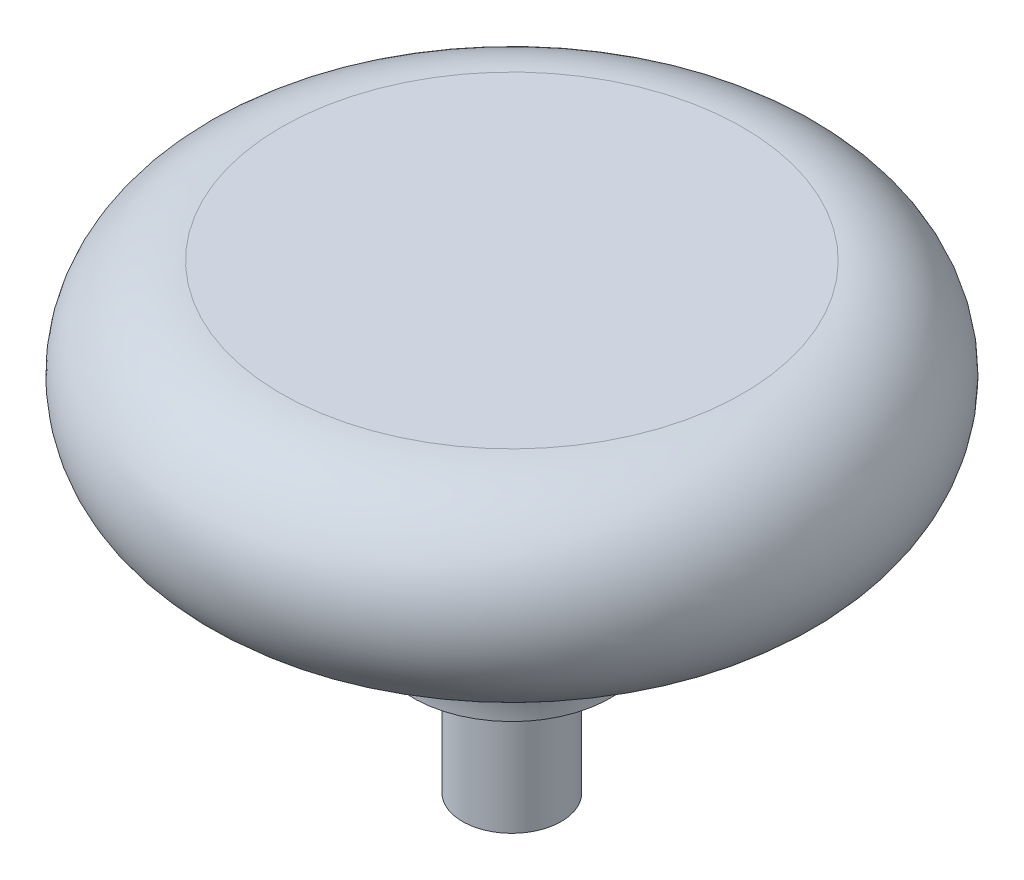
from build123d import *


with BuildPart() as part:
    # Knob Profile Sketch → Knob Body Revolve (revolve)
    with BuildSketch(Plane.XY, mode=Mode.PRIVATE) as knob_body_revolve_sk:
        with BuildLine():
            Line((0, 0), (2.38, 0))
            Line((2.38, 0), (2.38, 6.350001607))
            Line((2.38, 6.350001607), (4.765, 6.350001607))
            ThreePointArc((4.765, 6.350001607), (6.625882433, 10.841139934), (11.117857786, 12.700000964))
            ThreePointArc((11.117857786, 12.700000964), (15.88, 17.460000482), (11.117857786, 22.22))
            Line((11.117857786, 22.22), (0, 22.22))
            Line((0, 22.22), (0, 0))
        make_face()
    revolve(knob_body_revolve_sk.sketch.rotate(Axis((0, 22.22, 0), (0, -1, 0)), 180), axis=Axis((0, 22.22, 0), (0, -1, 0)))


solid = part.part
